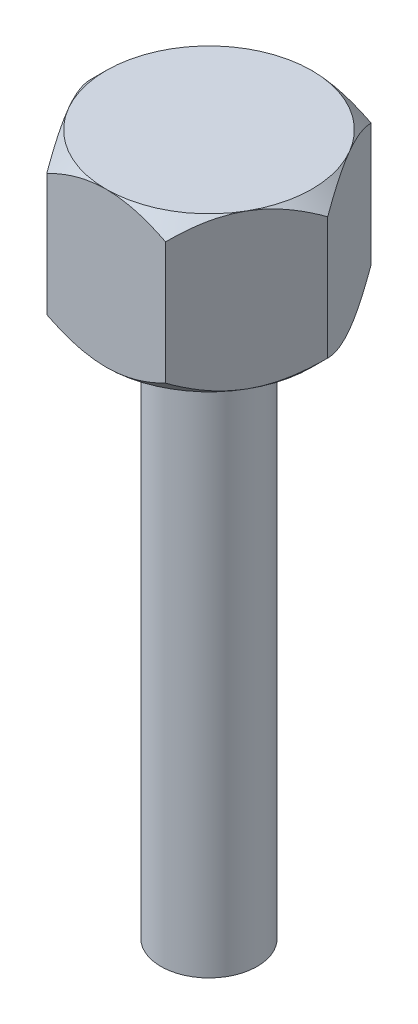
from build123d import *

# Parameters (mm, degrees)
HEX_HEAD_DEPTH                          = 6
HEAD_TOP_CHAMFER_SKETCH_OUTSIDE_W       = 29.96
HEAD_TOP_CHAMFER_SKETCH_OUTSIDE_H       = 28.722
HEAD_TOP_CHAMFER_SKETCH_OUTSIDE_R       = 4
HEAD_TOP_CHAMFER_45DEG_DEPTH            = 8
HEAD_TOP_CHAMFER_45DEG_DRAFT            = -45
SHANK_SKETCH_R                          = 1.875
SHANK_DEPTH                             = 21.25
HEAD_UNDERSIDE_CHAMFER_SKETCH_OUTSIDE_W = 59.71
HEAD_UNDERSIDE_CHAMFER_SKETCH_OUTSIDE_H = 58.472
HEAD_UNDERSIDE_CHAMFER_SKETCH_OUTSIDE_R = 4
HEAD_UNDERSIDE_CHAMFER_45DEG_DEPTH      = 21.25
HEAD_UNDERSIDE_CHAMFER_45DEG_DRAFT      = -45


with BuildPart() as part:
    # Hex Head Sketch → Hex Head (new body)
    with BuildSketch(Plane(origin=(0, 0, 0), x_dir=(1, 0, 0), z_dir=(0, 1, 0))):
        Polygon((-2.309401077, -4), (2.309401077, -4), (4.618802154, 0), (2.309401077, 4), (-2.309401077, 4), (-4.618802154, 0), align=None)
    extrude(amount=HEX_HEAD_DEPTH)


with BuildPart() as head_top_chamfer_45deg_tool:
    # Head Top Chamfer Sketch outside → Head Top Chamfer 45deg (with draft: the straight prism first)
    with BuildSketch(Plane(origin=(0, 6, 0), x_dir=(1, 0, 0), z_dir=(0, 1, 0))):
        Rectangle(HEAD_TOP_CHAMFER_SKETCH_OUTSIDE_W, HEAD_TOP_CHAMFER_SKETCH_OUTSIDE_H)
        Circle(HEAD_TOP_CHAMFER_SKETCH_OUTSIDE_R, mode=Mode.SUBTRACT)
    extrude(amount=-HEAD_TOP_CHAMFER_45DEG_DEPTH)
    # Head Top Chamfer 45deg: the draft: its side faces are tilted about the plane it starts from
    head_top_chamfer_45deg_sides = [head_top_chamfer_45deg_tool.faces().sort_by_distance(p)[0] for p in [
        (0, 2, 14.361),
        (14.98, 2, 0),
        (0, 2, -14.361),
        (-14.98, 2, 0),
        (-4, 2, 0),
    ]]
    draft(head_top_chamfer_45deg_sides, Plane(origin=(0, 6, 0), x_dir=(1, 0, 0), z_dir=(0, 1, 0)), HEAD_TOP_CHAMFER_45DEG_DRAFT)


with BuildPart() as part_1:
    add(part.part)

    # Head Top Chamfer 45deg: cut by head_top_chamfer_45deg_tool
    add(head_top_chamfer_45deg_tool.part, mode=Mode.SUBTRACT)

    # Shank Sketch → Shank (add)
    with BuildSketch(Plane.XZ):
        with Locations(Location((0, 0, 0), (0, 0, 270))):
            Circle(SHANK_SKETCH_R)
    extrude(amount=SHANK_DEPTH)


with BuildPart() as head_underside_chamfer_45deg_tool:
    # Head Underside Chamfer Sketch outside → Head Underside Chamfer 45deg (with draft: the straight prism first)
    with BuildSketch(Plane.XZ):
        Rectangle(HEAD_UNDERSIDE_CHAMFER_SKETCH_OUTSIDE_W, HEAD_UNDERSIDE_CHAMFER_SKETCH_OUTSIDE_H)
        Circle(HEAD_UNDERSIDE_CHAMFER_SKETCH_OUTSIDE_R, mode=Mode.SUBTRACT)
    extrude(amount=-HEAD_UNDERSIDE_CHAMFER_45DEG_DEPTH)
    # Head Underside Chamfer 45deg: the draft: its side faces are tilted about the plane it starts from
    head_underside_chamfer_45deg_sides = [head_underside_chamfer_45deg_tool.faces().sort_by_distance(p)[0] for p in [
        (0, 10.625, -29.236),
        (29.855, 10.625, 0),
        (0, 10.625, 29.236),
        (-29.855, 10.625, 0),
        (-4, 10.625, 0),
    ]]
    draft(head_underside_chamfer_45deg_sides, Plane.XZ, HEAD_UNDERSIDE_CHAMFER_45DEG_DRAFT)


with BuildPart() as part_2:
    add(part_1.part)

    # Head Underside Chamfer 45deg: cut by head_underside_chamfer_45deg_tool
    add(head_underside_chamfer_45deg_tool.part, mode=Mode.SUBTRACT)


solid = part_2.part
